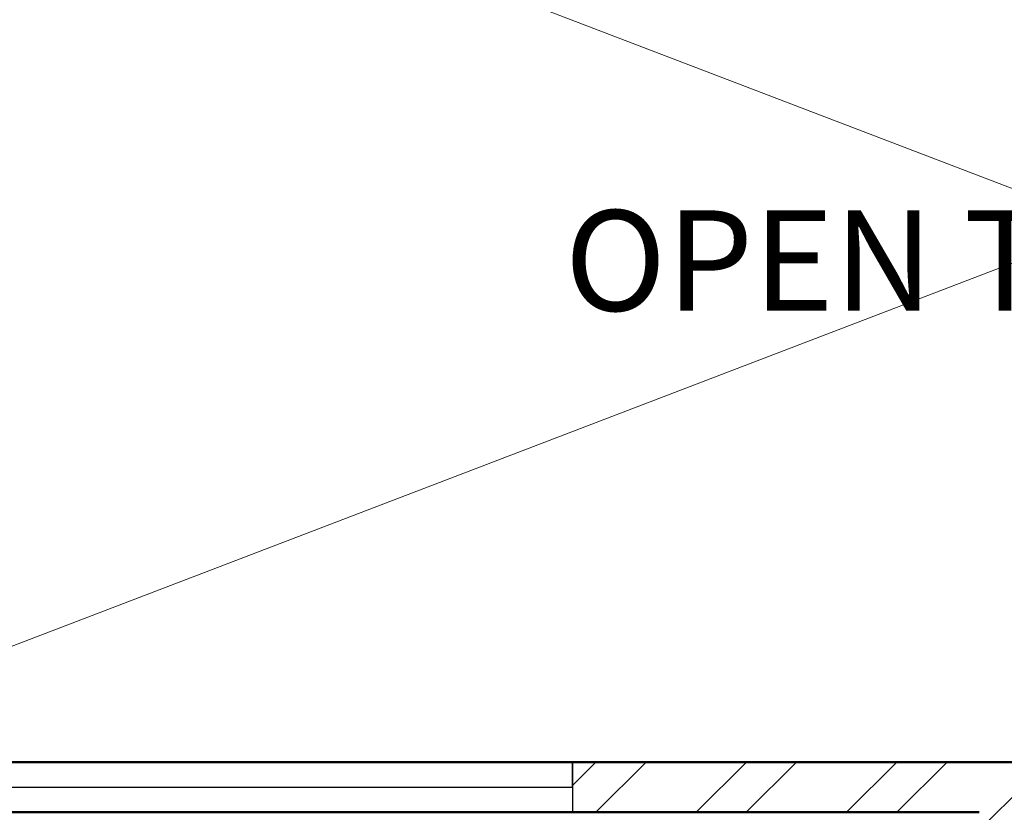
# Model space of a CAD drawing. Units: inches. Extents: x 1901 to 2863, y 888 to 2433.
# Tile 39 of 91: x 2530 to 2618, y 1661 to 1732. Entities that reach past the tile are written whole.
import ezdxf

# ---------------------------------------------------------------- set-up
doc = ezdxf.new("R2010")
doc.units = ezdxf.units.IN
for name, color, linetype, lineweight in [('A-ANNO-SYMB', 8, 'Continuous', 13), ('A-AREA-IDEN', 7, 'Continuous', 18), ('A-GLAZ', 3, 'Continuous', 25), ('A-WALL', 7, 'Continuous', 50), ('A-WALL-PATT', 8, 'Continuous', 13)]:
    doc.layers.add(name, color=color, linetype=linetype, lineweight=lineweight)
doc.styles.get("Standard").update_dxf_attribs({"font": 'arial.ttf'})

# ---------------------------------------------------------------- blocks, each defined once
blk = doc.blocks.new('WIN-60')
for p, q in [((0, 4.5), (0, 0)), ((60, 2.25), (60, 4.5)), ((60, 4.5), (60, 0)), ((0, 0), (0, 2.25)), ((0, 2.25), (60, 2.25))]:
    blk.add_line(p, q)

msp = doc.modelspace()

# ---------------------------------------------------------------- hatches: boundary and pattern name
at = {"layer": 'A-WALL-PATT'}
h = msp.add_hatch(dxfattribs=at)
h.set_pattern_fill('ANSI32', color=256)
h.paths.add_polyline_path([(2192.501, 2274.134), (2141.264, 2274.134), (2141.264, 2269.634), (2192.501, 2269.634)])
h.paths.add_polyline_path([(2259.926, 2274.134), (2216.501, 2274.134), (2216.501, 2269.634), (2255.426, 2269.634), (2255.426, 2214.634), (2250.809, 2214.634), (2250.809, 2210.134), (2259.926, 2210.134), (2259.926, 2215.134), (2271.756, 2215.134), (2271.756, 2217.384), (2271.756, 2219.634), (2259.926, 2219.634)])
h.paths.add_polyline_path([(2171.426, 2269.634), (2166.926, 2269.634), (2166.926, 2219.634), (2121.238, 2219.634), (2121.238, 2215.134), (2166.926, 2215.134), (2166.926, 2083.134), (2161.807, 2083.134), (2161.807, 2078.634), (2171.426, 2078.634), (2176.996, 2078.634), (2176.996, 2080.884), (2176.996, 2083.134), (2171.426, 2083.134), (2171.426, 2210.134), (2230.912, 2210.134), (2230.912, 2212.384), (2230.912, 2214.634), (2171.426, 2214.634)])
h.paths.add_polyline_path([(2117.264, 2274.134), (2089.426, 2274.134), (2089.426, 2219.634), (2081.136, 2219.634), (2081.136, 2215.134), (2089.426, 2215.134), (2098.004, 2215.134), (2098.004, 2217.384), (2098.004, 2219.634), (2093.926, 2219.634), (2093.926, 2269.634), (2117.264, 2269.634), (2117.264, 2271.884)])
h.paths.add_polyline_path([(2343.426, 2219.634), (2329.295, 2219.634), (2329.295, 2215.134), (2338.926, 2215.134), (2338.926, 2184.739), (2343.426, 2184.739)])
h.paths.add_polyline_path([(2338.926, 2083.134), (2329.295, 2083.134), (2208.966, 2083.134), (2208.966, 2078.634), (2338.926, 2078.634)])
h.paths.add_polyline_path([(2343.426, 2136.739), (2338.926, 2136.739), (2338.926, 1872.634), (2343.426, 1872.634)])
h.paths.add_polyline_path([(2343.426, 1863.634), (2397.68, 1863.634), (2397.68, 1821.634), (2384.138, 1821.634), (2384.138, 1812.634), (2418.33, 1812.634), (2418.33, 1817.134), (2418.33, 1821.634), (2406.68, 1821.634), (2406.68, 1863.634), (2459.499, 1863.634), (2459.499, 1821.634), (2447.138, 1821.634), (2447.138, 1812.634), (2459.499, 1812.634), (2468.499, 1812.634), (2468.499, 1872.634), (2394.426, 1872.634), (2334.426, 1872.634), (2334.426, 1812.634), (2343.426, 1812.634), (2353.251, 1812.634), (2353.251, 1821.634), (2343.426, 1821.634)])
h.paths.add_polyline_path([(2510.014, 1872.634), (2468.499, 1872.634), (2468.499, 1868.134), (2510.014, 1868.134)])
h.paths.add_polyline_path([(2514.009, 1817.134), (2468.499, 1817.134), (2468.499, 1812.634), (2482.114, 1812.634), (2482.114, 1800.606), (2486.614, 1800.606), (2486.614, 1812.634), (2514.009, 1812.634)])
h.paths.add_polyline_path([(2299.247, 1814.884), (2299.247, 1817.134), (2295.926, 1817.134), (2295.926, 1854.169), (2293.676, 1854.169), (2291.426, 1854.169), (2291.426, 1817.134), (2266.109, 1817.134), (2266.109, 1812.634), (2299.247, 1812.634)])
h.paths.add_polyline_path([(2218.109, 1817.134), (2206.46, 1817.134), (2171.426, 1817.134), (2171.426, 1949.134), (2190.1, 1949.134), (2190.1, 1953.634), (2163.468, 1953.634), (2163.468, 1949.134), (2166.926, 1949.134), (2166.926, 1817.134), (2114.297, 1817.134), (2114.297, 1812.634), (2218.109, 1812.634)])
h.paths.add_polyline_path([(2029.426, 1970.922), (2024.926, 1970.922), (2024.926, 1912.717), (2029.426, 1912.717)])
h.paths.add_polyline_path([(2132.297, 1953.634), (2113.926, 1953.634), (2113.926, 1975.888), (2111.676, 1975.888), (2109.426, 1975.888), (2109.426, 1953.634), (2029.426, 1953.634), (2029.426, 1949.134), (2132.297, 1949.134)])
h.paths.add_polyline_path([(2029.426, 1853.606), (2029.31, 1853.606), (2029.31, 1853.606), (2029.426, 1853.606), (2029.426, 1864.717), (2024.926, 1864.717), (2024.926, 1812.634), (2066.297, 1812.634), (2066.297, 1814.884), (2066.297, 1817.134), (2029.426, 1817.134)])
h.paths.add_polyline_path([(2122.926, 2010.088), (2120.676, 2010.088), (2118.426, 2010.088), (2118.426, 2006.134), (2029.426, 2006.134), (2029.426, 2001.634), (2109.426, 2001.634), (2109.426, 1998.041), (2113.926, 1998.041), (2113.926, 2001.634), (2122.926, 2001.634)])
h.paths.add_polyline_path([(2029.426, 2031.376), (2024.926, 2031.376), (2024.926, 1994.922), (2027.176, 1994.922), (2029.426, 1994.922)])
h.paths.add_polyline_path([(2029.426, 2136.739), (2024.926, 2136.739), (2024.926, 2067.376), (2027.176, 2067.376), (2029.426, 2067.376)])
h.paths.add_polyline_path([(2125.618, 2083.134), (2029.426, 2083.134), (2029.426, 2078.634), (2118.426, 2078.634), (2118.426, 2030.715), (2122.926, 2030.715), (2122.926, 2078.634), (2125.618, 2078.634)])
h.paths.add_polyline_path([(2029.426, 2215.134), (2040.468, 2215.134), (2040.468, 2217.384), (2040.468, 2219.634), (2024.926, 2219.634), (2024.926, 2184.739), (2029.426, 2184.739), (2029.426, 2187.778)])
h.paths.add_polyline_path([(2686.426, 2274.134), (2659.284, 2274.134), (2659.284, 2269.634), (2681.926, 2269.634), (2681.926, 2219.634), (2676.816, 2219.634), (2676.816, 2215.134), (2681.926, 2215.134), (2697.011, 2215.134), (2697.011, 2217.384), (2697.011, 2219.634), (2686.426, 2219.634)])
h.paths.add_polyline_path([(2609.926, 2269.634), (2635.284, 2269.634), (2635.284, 2274.134), (2571.431, 2274.134), (2571.431, 2269.634), (2605.426, 2269.634), (2605.426, 2214.634), (2549.098, 2214.634), (2549.098, 2210.134), (2605.426, 2210.134), (2605.426, 2083.134), (2601.014, 2083.134), (2601.014, 2080.884), (2601.014, 2078.634), (2609.926, 2078.634), (2616.162, 2078.634), (2616.162, 2080.884), (2616.162, 2083.134), (2609.926, 2083.134), (2609.926, 2215.134), (2651.465, 2215.134), (2651.465, 2217.384), (2651.465, 2219.634), (2609.926, 2219.634)])
h.paths.add_polyline_path([(2521.426, 2269.634), (2547.431, 2269.634), (2547.431, 2271.884), (2547.431, 2274.134), (2516.926, 2274.134), (2516.926, 2219.634), (2506.41, 2219.634), (2506.41, 2215.134), (2516.926, 2215.134), (2516.926, 2210.134), (2525.402, 2210.134), (2525.402, 2212.384), (2525.402, 2214.634), (2521.426, 2214.634)])
h.paths.add_polyline_path([(2456.011, 2219.634), (2439.426, 2219.634), (2439.426, 2187.888), (2443.926, 2187.888), (2443.926, 2215.134), (2456.011, 2215.134)])
h.paths.add_polyline_path([(2752.926, 2219.634), (2739.485, 2219.634), (2739.485, 2215.134), (2748.426, 2215.134), (2748.426, 2187.888), (2752.926, 2187.888)])
h.paths.add_polyline_path([(2752.926, 2139.888), (2748.426, 2139.888), (2748.426, 2083.134), (2648.416, 2083.134), (2648.416, 2078.634), (2654.926, 2078.634), (2654.926, 2039.437), (2659.426, 2039.437), (2659.426, 2078.634), (2748.426, 2078.634), (2748.426, 2063.429), (2752.926, 2063.429)])
h.paths.add_polyline_path([(2752.926, 2010.634), (2659.426, 2010.634), (2659.426, 2015.652), (2654.926, 2015.652), (2654.926, 2010.634), (2605.426, 2010.634), (2605.426, 1920.967), (2609.926, 1920.967), (2609.926, 2006.134), (2748.426, 2006.134), (2748.426, 1982.466), (2752.926, 1982.466)])
h.paths.add_polyline_path([(2752.926, 2027.429), (2748.426, 2027.429), (2748.426, 2010.634), (2752.926, 2010.634)])
h.paths.add_polyline_path([(2748.426, 1886.134), (2609.926, 1886.134), (2609.926, 1889.719), (2605.426, 1889.719), (2605.426, 1861.262), (2609.926, 1861.262), (2609.926, 1881.634), (2748.426, 1881.634)])
h.paths.add_polyline_path([(2456.855, 2228.831), (2498.401, 2228.831), (2498.401, 2247.488), (2456.855, 2247.488)], flags=9)
h.paths.add_polyline_path([(2038.602, 2237.418), (2080.174, 2237.418), (2080.174, 2256.075), (2038.602, 2256.075)], flags=9)
h.paths.add_polyline_path([(2292.009, 1062.394), (2539.932, 1062.394), (2539.932, 1099.487), (2292.009, 1099.487)], flags=9)
h.paths.add_polyline_path([(2424.91, 1832.253), (2448.513, 1832.253), (2448.513, 1846.678), (2424.91, 1846.678)], flags=25)
h.paths.add_polyline_path([(2359.076, 1832.253), (2382.678, 1832.253), (2382.678, 1846.678), (2359.076, 1846.678)], flags=25)
h.paths.add_polyline_path([(2352.899, 1684.802), (2367.543, 1684.802), (2367.543, 1697.167), (2352.899, 1697.167)], flags=9)
h.paths.add_polyline_path([(2079.288, 1755.826), (2169.024, 1755.826), (2169.024, 1774.372), (2079.288, 1774.372)], flags=9)
h.paths.add_polyline_path([(2404.09, 1373.857), (2404.09, 1463.593), (2385.544, 1463.593), (2385.544, 1373.857)], flags=9)
h.paths.add_polyline_path([(2268.091, 2236.371), (2309.636, 2236.371), (2309.636, 2255.028), (2268.091, 2255.028)], flags=9)
h.paths.add_polyline_path([(2575.96, 1700.951), (2665.696, 1700.951), (2665.696, 1719.498), (2575.96, 1719.498)], flags=9)
h.paths.add_polyline_path([(2302.962, 1878.474), (2329.524, 1878.474), (2329.524, 1888.777), (2302.962, 1888.777)], flags=9)
h.paths.add_polyline_path([(2097.415, 2240.576), (2126.573, 2240.576), (2126.573, 2259.233), (2097.415, 2259.233)], flags=9)
h.paths.add_polyline_path([(2208.725, 2246.124), (2237.882, 2246.124), (2237.882, 2264.781), (2208.725, 2264.781)], flags=9)
h.paths.add_polyline_path([(2038.147, 1925.958), (2076.987, 1925.958), (2076.987, 1944.615), (2038.147, 1944.615)], flags=9)
h.paths.add_polyline_path([(2239.144, 1926.672), (2288.465, 1926.672), (2288.465, 1945.329), (2239.144, 1945.329)], flags=9)
h.paths.add_polyline_path([(2175.429, 2007.33), (2212.356, 2007.33), (2212.356, 2025.987), (2175.429, 2025.987)], flags=9)
h.paths.add_polyline_path([(2225.034, 2091.794), (2263.875, 2091.794), (2263.875, 2110.451), (2225.034, 2110.451)], flags=9)
h.paths.add_polyline_path([(2035.398, 2098.478), (2074.238, 2098.478), (2074.238, 2117.135), (2035.398, 2117.135)], flags=9)
h.paths.add_polyline_path([(2050.102, 2029.209), (2083.26, 2029.209), (2083.26, 2047.866), (2050.102, 2047.866)], flags=9)
h.paths.add_polyline_path([(2069.677, 1956.719), (2098.835, 1956.719), (2098.835, 1975.376), (2069.677, 1975.376)], flags=25)
h.paths.add_polyline_path([(2328.62, 1753.336), (2361.663, 1753.336), (2361.663, 1771.993), (2328.62, 1771.993)], flags=9)
h.paths.add_polyline_path([(2395.162, 2060.888), (2395.162, 2140.654), (2378.676, 2140.654), (2378.676, 2060.888)], flags=9)
h.paths.add_polyline_path([(2463.728, 2059.02), (2492.886, 2059.02), (2492.886, 2077.677), (2463.728, 2077.677)], flags=9)
h.paths.add_polyline_path([(2458.027, 2181.536), (2496.868, 2181.536), (2496.868, 2200.194), (2458.027, 2200.194)], flags=9)
h.paths.add_polyline_path([(2527.577, 2243.074), (2556.735, 2243.074), (2556.735, 2261.731), (2527.577, 2261.731)], flags=9)
h.paths.add_polyline_path([(2694.461, 2232.767), (2736.033, 2232.767), (2736.033, 2251.425), (2694.461, 2251.425)], flags=9)
h.paths.add_polyline_path([(2637.821, 2249.225), (2666.979, 2249.225), (2666.979, 2267.882), (2637.821, 2267.882)], flags=9)
h.paths.add_polyline_path([(2623.687, 2183.541), (2662.528, 2183.541), (2662.528, 2202.199), (2623.687, 2202.199)], flags=9)
h.paths.add_polyline_path([(2691.965, 2021.5), (2725.124, 2021.5), (2725.124, 2040.157), (2691.965, 2040.157)], flags=9)
h.paths.add_polyline_path([(2621.043, 1975.912), (2662.335, 1975.912), (2662.335, 1994.569), (2621.043, 1994.569)], flags=25)
h.paths.add_polyline_path([(2479.032, 1927.62), (2519.844, 1927.62), (2519.844, 1946.277), (2479.032, 1946.277)], flags=9)
h.paths.add_polyline_path([(2670.941, 1849.076), (2716.005, 1849.076), (2716.005, 1867.734), (2670.941, 1867.734)], flags=9)
h.paths.add_polyline_path([(2523.613, 1782.956), (2550.175, 1782.956), (2550.175, 1793.26), (2523.613, 1793.26)], flags=9)
h.paths.add_polyline_path([(2450.841, 1207.331), (2492.386, 1207.331), (2492.386, 1225.989), (2450.841, 1225.989)], flags=9)
h.paths.add_polyline_path([(2527.751, 1203.841), (2556.908, 1203.841), (2556.908, 1222.499), (2527.751, 1222.499)], flags=9)
h.paths.add_polyline_path([(2639.111, 1207.2), (2668.268, 1207.2), (2668.268, 1225.857), (2639.111, 1225.857)], flags=9)
h.paths.add_polyline_path([(2692.594, 1218.965), (2734.167, 1218.965), (2734.167, 1237.623), (2692.594, 1237.623)], flags=9)
h.paths.add_polyline_path([(2669.266, 1366.329), (2708.106, 1366.329), (2708.106, 1384.987), (2669.266, 1384.987)], flags=9)
h.paths.add_polyline_path([(2463.313, 1358.031), (2502.153, 1358.031), (2502.153, 1376.688), (2463.313, 1376.688)], flags=9)
h.paths.add_polyline_path([(2494.725, 1449.963), (2531.652, 1449.963), (2531.652, 1468.62), (2494.725, 1468.62)], flags=9)
h.paths.add_polyline_path([(2675.565, 1422.157), (2708.724, 1422.157), (2708.724, 1440.815), (2675.565, 1440.815)], flags=9)
h.paths.add_polyline_path([(2685.634, 1493.891), (2714.792, 1493.891), (2714.792, 1512.548), (2685.634, 1512.548)], flags=9)
h.paths.add_polyline_path([(2686.805, 1529.913), (2725.645, 1529.913), (2725.645, 1548.57), (2686.805, 1548.57)], flags=9)
h.paths.add_polyline_path([(2503.651, 1537.991), (2552.972, 1537.991), (2552.972, 1556.648), (2503.651, 1556.648)], flags=9)
h.paths.add_polyline_path([(2291.713, 1643.504), (2318.275, 1643.504), (2318.275, 1653.807), (2291.713, 1653.807)], flags=9)
h.paths.add_polyline_path([(2450.626, 1610.52), (2477.189, 1610.52), (2477.189, 1620.824), (2450.626, 1620.824)], flags=9)
h.paths.add_polyline_path([(2359.985, 1551.814), (2422.253, 1551.814), (2422.253, 1562.117), (2359.985, 1562.117)], flags=9)
h.paths.add_polyline_path([(2280.106, 1249.006), (2321.651, 1249.006), (2321.651, 1267.663), (2280.106, 1267.663)], flags=9)
h.paths.add_polyline_path([(2164.057, 1274.232), (2193.215, 1274.232), (2193.215, 1292.889), (2164.057, 1292.889)], flags=9)
h.paths.add_polyline_path([(2118.21, 1277.694), (2151.252, 1277.694), (2151.252, 1296.351), (2118.21, 1296.351)], flags=9)
h.paths.add_polyline_path([(2031.946, 1268.529), (2073.519, 1268.529), (2073.519, 1287.187), (2031.946, 1287.187)], flags=9)
h.paths.add_polyline_path([(2050.199, 1409.079), (2089.04, 1409.079), (2089.04, 1427.736), (2050.199, 1427.736)], flags=9)
h.paths.add_polyline_path([(2243.743, 1421.032), (2282.584, 1421.032), (2282.584, 1439.689), (2243.743, 1439.689)], flags=9)
h.paths.add_polyline_path([(2190.746, 1509.769), (2231.558, 1509.769), (2231.558, 1528.426), (2190.746, 1528.426)], flags=9)
h.paths.add_polyline_path([(2058.392, 1475.415), (2091.55, 1475.415), (2091.55, 1494.073), (2058.392, 1494.073)], flags=9)
h.paths.add_polyline_path([(2062.447, 1553.09), (2091.605, 1553.09), (2091.605, 1571.747), (2062.447, 1571.747)], flags=9)
h.paths.add_polyline_path([(2219.524, 1590.365), (2266.147, 1590.365), (2266.147, 1609.022), (2219.524, 1609.022)], flags=9)
h.paths.add_polyline_path([(2041.072, 1584.188), (2079.912, 1584.188), (2079.912, 1602.845), (2041.072, 1602.845)], flags=9)
h = msp.add_hatch(dxfattribs=at)
h.set_pattern_fill('ANSI32', color=256)
h.paths.add_polyline_path([(2443.926, 2139.888), (2439.426, 2139.888), (2439.426, 2069.348), (2441.676, 2069.348), (2443.926, 2069.348), (2443.926, 2078.634), (2521.926, 2078.634), (2521.926, 2075.067), (2524.176, 2075.067), (2526.426, 2075.067), (2526.426, 2078.634), (2571.755, 2078.634), (2571.755, 2080.884), (2571.755, 2083.134), (2443.926, 2083.134)])
h.paths.add_polyline_path([(2526.426, 2054.634), (2524.176, 2054.634), (2521.926, 2054.634), (2521.926, 2030.634), (2443.926, 2030.634), (2443.926, 2045.348), (2439.426, 2045.348), (2439.426, 1983.867), (2443.926, 1983.867), (2443.926, 2026.134), (2521.926, 2026.134), (2526.426, 2026.134)])
h.paths.add_polyline_path([(2443.926, 1923.867), (2439.426, 1923.867), (2439.426, 1872.634), (2443.926, 1872.634)])
h.paths.add_polyline_path([(2636.233, 1766.134), (2609.926, 1766.134), (2609.926, 1779.785), (2605.426, 1779.785), (2605.426, 1766.134), (2486.614, 1766.134), (2486.614, 1770.671), (2482.114, 1770.671), (2482.114, 1766.134), (2482.114, 1761.634), (2636.233, 1761.634), (2636.233, 1763.884)])
h.paths.add_polyline_path([(2519.536, 1663.384), (2519.536, 1665.634), (2494.926, 1665.634), (2481.831, 1665.634), (2481.831, 1663.384), (2481.831, 1661.134), (2490.426, 1661.134), (2490.426, 1640.157), (2494.926, 1640.157), (2494.926, 1661.134), (2519.536, 1661.134)])
h.paths.add_polyline_path([(2443.926, 1712.134), (2443.926, 1716.634), (2414.464, 1716.634), (2414.464, 1712.134), (2439.426, 1712.134), (2439.426, 1545.507), (2443.926, 1545.507), (2443.926, 1661.134), (2448.475, 1661.134), (2448.475, 1665.634), (2443.926, 1665.634)])
h.paths.add_polyline_path([(2343.426, 1712.134), (2365.525, 1712.134), (2365.525, 1714.384), (2365.525, 1716.634), (2333.871, 1716.634), (2333.871, 1714.384), (2333.871, 1712.134), (2338.926, 1712.134), (2338.926, 1575.634), (2338.926, 1545.507), (2343.426, 1545.507), (2343.426, 1547.507), (2343.426, 1580.134)])
h.paths.add_polyline_path([(2752.926, 1665.634), (2579.536, 1665.634), (2579.536, 1661.134), (2615.926, 1661.134), (2615.926, 1529.134), (2598.931, 1529.134), (2598.931, 1524.634), (2623.127, 1524.634), (2623.127, 1526.884), (2623.127, 1529.134), (2620.426, 1529.134), (2620.426, 1661.134), (2748.426, 1661.134), (2748.426, 1633.499), (2752.926, 1633.499)])
h.paths.add_polyline_path([(2752.926, 1419.929), (2748.426, 1419.929), (2748.426, 1400.134), (2659.426, 1400.134), (2659.426, 1444.333), (2657.176, 1444.333), (2654.926, 1444.333), (2654.926, 1400.134), (2643.649, 1400.134), (2643.649, 1395.634), (2748.426, 1395.634), (2748.426, 1364.035), (2752.926, 1364.035)])
h.paths.add_polyline_path([(2752.926, 1492.878), (2748.426, 1492.878), (2748.426, 1476.634), (2667.426, 1476.634), (2667.426, 1479.71), (2665.176, 1479.71), (2662.926, 1479.71), (2662.926, 1476.634), (2654.926, 1476.634), (2654.926, 1469.536), (2659.426, 1469.536), (2659.426, 1472.134), (2748.426, 1472.134), (2748.426, 1455.929), (2752.926, 1455.929)])
h.paths.add_polyline_path([(2752.926, 1304.035), (2748.426, 1304.035), (2748.426, 1263.634), (2738.66, 1263.634), (2738.66, 1259.134), (2752.926, 1259.134)])
h.paths.add_polyline_path([(2685.926, 1259.134), (2695.49, 1259.134), (2695.49, 1261.384), (2695.49, 1263.634), (2677.837, 1263.634), (2677.837, 1261.384), (2677.837, 1259.134), (2681.426, 1259.134), (2681.426, 1203.634), (2653.277, 1203.634), (2653.277, 1199.134), (2685.926, 1199.134), (2685.926, 1203.634)])
h.paths.add_polyline_path([(2609.426, 1395.634), (2611.848, 1395.634), (2611.848, 1400.134), (2598.888, 1400.134), (2598.888, 1397.884), (2598.888, 1395.634), (2604.926, 1395.634), (2604.926, 1268.134), (2554.726, 1268.134), (2554.726, 1265.884), (2554.726, 1263.634), (2604.926, 1263.634), (2604.926, 1203.634), (2571.306, 1203.634), (2571.306, 1199.134), (2604.926, 1199.134), (2629.277, 1199.134), (2629.277, 1201.384), (2629.277, 1203.634), (2609.426, 1203.634), (2609.426, 1258.634), (2609.426, 1259.134), (2654.804, 1259.134), (2654.804, 1263.634), (2609.426, 1263.634)])
h.paths.add_polyline_path([(2443.926, 1304.035), (2439.426, 1304.035), (2439.426, 1259.134), (2443.926, 1259.134), (2456.16, 1259.134), (2456.16, 1261.384), (2456.16, 1263.634), (2443.926, 1263.634)])
h.paths.add_polyline_path([(2525.426, 1263.634), (2531.778, 1263.634), (2531.778, 1268.134), (2520.926, 1268.134), (2520.926, 1263.634), (2511.409, 1263.634), (2511.409, 1259.134), (2520.926, 1259.134), (2520.926, 1199.134), (2547.306, 1199.134), (2547.306, 1201.384), (2547.306, 1203.634), (2525.426, 1203.634)])
h.paths.add_polyline_path([(2443.926, 1434.842), (2439.426, 1434.842), (2439.426, 1364.035), (2441.676, 1364.035), (2443.926, 1364.035)])
h.paths.add_polyline_path([(2567.134, 1400.134), (2443.926, 1400.134), (2443.926, 1395.634), (2567.134, 1395.634)])
h.paths.add_polyline_path([(2443.926, 1545.507), (2439.426, 1545.507), (2439.426, 1494.842), (2443.926, 1494.842)])
h.paths.add_polyline_path([(2494.926, 1553.349), (2492.676, 1553.349), (2490.426, 1553.349), (2490.426, 1524.634), (2494.926, 1524.634), (2525.936, 1524.634), (2525.936, 1526.884), (2525.936, 1529.134), (2494.926, 1529.134)])
h.paths.add_polyline_path([(2752.926, 1573.499), (2748.426, 1573.499), (2748.426, 1529.134), (2657.759, 1529.134), (2657.759, 1524.634), (2662.926, 1524.634), (2662.926, 1498.631), (2667.426, 1498.631), (2667.426, 1524.634), (2748.426, 1524.634), (2748.426, 1516.878), (2752.926, 1516.878)])
h.paths.add_polyline_path([(2038.602, 2237.418), (2080.174, 2237.418), (2080.174, 2256.075), (2038.602, 2256.075)], flags=9)
h.paths.add_polyline_path([(2292.009, 1062.394), (2539.932, 1062.394), (2539.932, 1099.487), (2292.009, 1099.487)], flags=9)
h.paths.add_polyline_path([(2424.91, 1832.253), (2448.513, 1832.253), (2448.513, 1846.678), (2424.91, 1846.678)], flags=9)
h.paths.add_polyline_path([(2359.076, 1832.253), (2382.678, 1832.253), (2382.678, 1846.678), (2359.076, 1846.678)], flags=9)
h.paths.add_polyline_path([(2352.899, 1684.802), (2367.543, 1684.802), (2367.543, 1697.167), (2352.899, 1697.167)], flags=9)
h.paths.add_polyline_path([(2079.288, 1755.826), (2169.024, 1755.826), (2169.024, 1774.372), (2079.288, 1774.372)], flags=9)
h.paths.add_polyline_path([(2404.09, 1373.857), (2404.09, 1463.593), (2385.544, 1463.593), (2385.544, 1373.857)], flags=9)
h.paths.add_polyline_path([(2268.091, 2236.371), (2309.636, 2236.371), (2309.636, 2255.028), (2268.091, 2255.028)], flags=9)
h.paths.add_polyline_path([(2575.96, 1700.951), (2665.696, 1700.951), (2665.696, 1719.498), (2575.96, 1719.498)], flags=9)
h.paths.add_polyline_path([(2302.962, 1878.474), (2329.524, 1878.474), (2329.524, 1888.777), (2302.962, 1888.777)], flags=9)
h.paths.add_polyline_path([(2097.415, 2240.576), (2126.573, 2240.576), (2126.573, 2259.233), (2097.415, 2259.233)], flags=9)
h.paths.add_polyline_path([(2208.725, 2246.124), (2237.882, 2246.124), (2237.882, 2264.781), (2208.725, 2264.781)], flags=9)
h.paths.add_polyline_path([(2038.147, 1925.958), (2076.987, 1925.958), (2076.987, 1944.615), (2038.147, 1944.615)], flags=9)
h.paths.add_polyline_path([(2239.144, 1926.672), (2288.465, 1926.672), (2288.465, 1945.329), (2239.144, 1945.329)], flags=9)
h.paths.add_polyline_path([(2175.429, 2007.33), (2212.356, 2007.33), (2212.356, 2025.987), (2175.429, 2025.987)], flags=9)
h.paths.add_polyline_path([(2225.034, 2091.794), (2263.875, 2091.794), (2263.875, 2110.451), (2225.034, 2110.451)], flags=9)
h.paths.add_polyline_path([(2035.398, 2098.478), (2074.238, 2098.478), (2074.238, 2117.135), (2035.398, 2117.135)], flags=9)
h.paths.add_polyline_path([(2050.102, 2029.209), (2083.26, 2029.209), (2083.26, 2047.866), (2050.102, 2047.866)], flags=9)
h.paths.add_polyline_path([(2069.677, 1956.719), (2098.835, 1956.719), (2098.835, 1975.376), (2069.677, 1975.376)], flags=9)
h.paths.add_polyline_path([(2328.62, 1753.336), (2361.663, 1753.336), (2361.663, 1771.993), (2328.62, 1771.993)], flags=9)
h.paths.add_polyline_path([(2395.162, 2060.888), (2395.162, 2140.654), (2378.676, 2140.654), (2378.676, 2060.888)], flags=9)
h.paths.add_polyline_path([(2463.728, 2059.02), (2492.886, 2059.02), (2492.886, 2077.677), (2463.728, 2077.677)], flags=9)
h.paths.add_polyline_path([(2458.027, 2181.536), (2496.868, 2181.536), (2496.868, 2200.194), (2458.027, 2200.194)], flags=9)
h.paths.add_polyline_path([(2456.855, 2228.831), (2498.401, 2228.831), (2498.401, 2247.488), (2456.855, 2247.488)], flags=9)
h.paths.add_polyline_path([(2527.577, 2243.074), (2556.735, 2243.074), (2556.735, 2261.731), (2527.577, 2261.731)], flags=9)
h.paths.add_polyline_path([(2694.461, 2232.767), (2736.033, 2232.767), (2736.033, 2251.425), (2694.461, 2251.425)], flags=9)
h.paths.add_polyline_path([(2637.821, 2249.225), (2666.979, 2249.225), (2666.979, 2267.882), (2637.821, 2267.882)], flags=9)
h.paths.add_polyline_path([(2623.687, 2183.541), (2662.528, 2183.541), (2662.528, 2202.199), (2623.687, 2202.199)], flags=9)
h.paths.add_polyline_path([(2691.965, 2021.5), (2725.124, 2021.5), (2725.124, 2040.157), (2691.965, 2040.157)], flags=9)
h.paths.add_polyline_path([(2621.043, 1975.912), (2662.335, 1975.912), (2662.335, 1994.569), (2621.043, 1994.569)], flags=9)
h.paths.add_polyline_path([(2479.032, 1927.62), (2519.844, 1927.62), (2519.844, 1946.277), (2479.032, 1946.277)], flags=9)
h.paths.add_polyline_path([(2670.941, 1849.076), (2716.005, 1849.076), (2716.005, 1867.734), (2670.941, 1867.734)], flags=9)
h.paths.add_polyline_path([(2523.613, 1782.956), (2550.175, 1782.956), (2550.175, 1793.26), (2523.613, 1793.26)], flags=9)
h.paths.add_polyline_path([(2450.841, 1207.331), (2492.386, 1207.331), (2492.386, 1225.989), (2450.841, 1225.989)], flags=9)
h.paths.add_polyline_path([(2527.751, 1203.841), (2556.908, 1203.841), (2556.908, 1222.499), (2527.751, 1222.499)], flags=9)
h.paths.add_polyline_path([(2639.111, 1207.2), (2668.268, 1207.2), (2668.268, 1225.857), (2639.111, 1225.857)], flags=9)
h.paths.add_polyline_path([(2692.594, 1218.965), (2734.167, 1218.965), (2734.167, 1237.623), (2692.594, 1237.623)], flags=9)
h.paths.add_polyline_path([(2669.266, 1366.329), (2708.106, 1366.329), (2708.106, 1384.987), (2669.266, 1384.987)], flags=25)
h.paths.add_polyline_path([(2463.313, 1358.031), (2502.153, 1358.031), (2502.153, 1376.688), (2463.313, 1376.688)], flags=9)
h.paths.add_polyline_path([(2494.725, 1449.963), (2531.652, 1449.963), (2531.652, 1468.62), (2494.725, 1468.62)], flags=9)
h.paths.add_polyline_path([(2675.565, 1422.157), (2708.724, 1422.157), (2708.724, 1440.815), (2675.565, 1440.815)], flags=25)
h.paths.add_polyline_path([(2685.634, 1493.891), (2714.792, 1493.891), (2714.792, 1512.548), (2685.634, 1512.548)], flags=9)
h.paths.add_polyline_path([(2686.805, 1529.913), (2725.645, 1529.913), (2725.645, 1548.57), (2686.805, 1548.57)], flags=25)
h.paths.add_polyline_path([(2503.651, 1537.991), (2552.972, 1537.991), (2552.972, 1556.648), (2503.651, 1556.648)], flags=9)
h.paths.add_polyline_path([(2291.713, 1643.504), (2318.275, 1643.504), (2318.275, 1653.807), (2291.713, 1653.807)], flags=9)
h.paths.add_polyline_path([(2450.626, 1610.52), (2477.189, 1610.52), (2477.189, 1620.824), (2450.626, 1620.824)], flags=9)
h.paths.add_polyline_path([(2359.985, 1551.814), (2422.253, 1551.814), (2422.253, 1562.117), (2359.985, 1562.117)], flags=9)
h.paths.add_polyline_path([(2280.106, 1249.006), (2321.651, 1249.006), (2321.651, 1267.663), (2280.106, 1267.663)], flags=9)
h.paths.add_polyline_path([(2164.057, 1274.232), (2193.215, 1274.232), (2193.215, 1292.889), (2164.057, 1292.889)], flags=9)
h.paths.add_polyline_path([(2118.21, 1277.694), (2151.252, 1277.694), (2151.252, 1296.351), (2118.21, 1296.351)], flags=9)
h.paths.add_polyline_path([(2031.946, 1268.529), (2073.519, 1268.529), (2073.519, 1287.187), (2031.946, 1287.187)], flags=9)
h.paths.add_polyline_path([(2050.199, 1409.079), (2089.04, 1409.079), (2089.04, 1427.736), (2050.199, 1427.736)], flags=9)
h.paths.add_polyline_path([(2243.743, 1421.032), (2282.584, 1421.032), (2282.584, 1439.689), (2243.743, 1439.689)], flags=9)
h.paths.add_polyline_path([(2190.746, 1509.769), (2231.558, 1509.769), (2231.558, 1528.426), (2190.746, 1528.426)], flags=9)
h.paths.add_polyline_path([(2058.392, 1475.415), (2091.55, 1475.415), (2091.55, 1494.073), (2058.392, 1494.073)], flags=9)
h.paths.add_polyline_path([(2062.447, 1553.09), (2091.605, 1553.09), (2091.605, 1571.747), (2062.447, 1571.747)], flags=9)
h.paths.add_polyline_path([(2219.524, 1590.365), (2266.147, 1590.365), (2266.147, 1609.022), (2219.524, 1609.022)], flags=9)
h.paths.add_polyline_path([(2041.072, 1584.188), (2079.912, 1584.188), (2079.912, 1602.845), (2041.072, 1602.845)], flags=9)

# ---------------------------------------------------------------- linework, layer by layer
at = {"layer": 'A-ANNO-SYMB'}
for p, q in [((2502.242, 1761.634), (2752.926, 1665.634)), ((2752.926, 1761.634), (2502.242, 1665.634))]:
    msp.add_line(p, q, dxfattribs=at)
at = {"layer": 'A-WALL'}
for p, q in [((2752.926, 1665.634), (2481.831, 1665.634)), ((2615.926, 1665.634), (2494.926, 1665.634)), ((2494.926, 1661.134), (2615.926, 1661.134))]:
    msp.add_line(p, q, dxfattribs=at)

# ---------------------------------------------------------------- block references
at = {"layer": 'A-GLAZ'}
msp.add_blockref('WIN-60', (2519.535, 1661.134), dxfattribs=at)

# ---------------------------------------------------------------- texts
at = {"layer": 'A-AREA-IDEN', "insert": (2578.817, 1715.025), "char_height": 9, "attachment_point": 1}
msp.add_mtext_dynamic_manual_height_columns('OPEN TO SKY', width=233.33037, gutter_width=12.5, heights=[0], dxfattribs=at)

doc.saveas('drawing.dxf')
